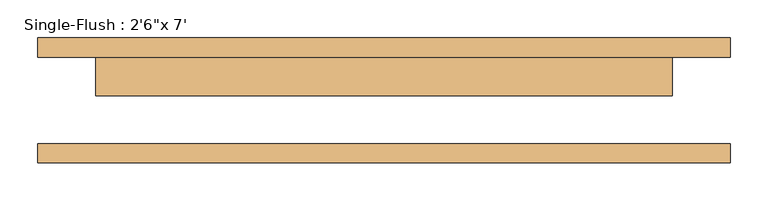
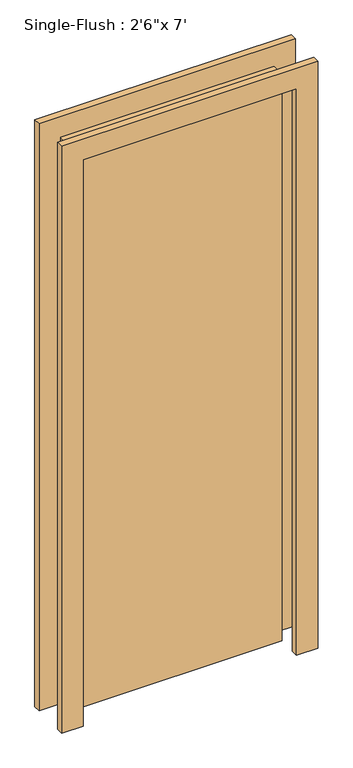
"""IFC4 building model written with IfcOpenShell, lengths in millimetres: door geometry."""

from ifc_helpers import new_model, si_unit, frame, origin, origin_with_axes, place, context, project, spatial, polyline, outline, extrude, source, transform, mapped, element, save


def door_214872d5(model_context):
    return source(origin(), model_context, "Body", "SweptSolid", [
        extrude(outline(polyline([(2209.8, -457.2), (0.0, -457.2), (0.0, -381.0), (2133.6, -381.0), (2133.6, 381.0), (0.0, 381.0), (0.0, 457.2), (2209.8, 457.2), (2209.8, -457.2)])), frame((0.0, 57.15, 0.0), z_axis=(0.0, 1.0, 0.0), x_axis=(0.0, 0.0, 1.0)), (0.0, 0.0, 1.0), 25.4),
        extrude(outline(polyline([(2209.8, 457.2), (2209.8, -457.2), (0.0, -457.2), (0.0, -381.0), (2133.6, -381.0), (2133.6, 381.0), (0.0, 381.0), (0.0, 457.2), (2209.8, 457.2)])), frame((0.0, -82.55, 0.0), z_axis=(0.0, 1.0, 0.0), x_axis=(0.0, 0.0, 1.0)), (0.0, 0.0, 1.0), 25.4),
        extrude(outline(polyline([(381.0, 6.35), (-381.0, 6.35), (-381.0, 57.15), (381.0, 57.15), (381.0, 6.35)])), origin_with_axes(), (0.0, 0.0, 1.0), 2133.6),
    ])


if __name__ == "__main__":
    model = new_model("IFC4")
    model_context = context("Model", 3, world=origin())
    ifc_project = project(units=[si_unit("LENGTHUNIT", "METRE", prefix="MILLI")], contexts=[model_context])
    site = spatial("IfcSite", under=ifc_project)
    building = spatial("IfcBuilding", under=site)
    placement = place(None, origin())
    door_shape = door_214872d5(model_context)
    element("IfcDoor", 1, ObjectType="Single-Flush : 2'6\"x 7'", at=placement, inside=building, context=model_context, shape_type="MappedRepresentation", body=[
        mapped(door_shape, transform((0.0, 0.0, 0.0), x_axis=(1.0, 0.0, 0.0), y_axis=(0.0, 1.0, 0.0), z_axis=(0.0, 0.0, 1.0))),
    ])
    save(model, "model.ifc")

# Revit data of these elements
# Type "Single-Flush : 2'6\"x 7'"
#   Type Mark = "8"
#   Construction Type Id = "MDOOR"
#   Assembly Code = "C1020"
#   Analytic Construction = "Metal"
#   Thickness = 0' - 2"
#   Heat Transfer Coefficient (U) = 0.651978 BTU/(h·ft²·°F)
#   Height = 7' - 0"
#   Trim Projection Ext = 0' - 1"
#   Trim Projection Int = 0' - 1"
#   Trim Width = 0' - 3"
#   Width = 2' - 6"
#   Define Thermal Properties by = 1
#   Door Material = Door - Panel
#   Frame Material = Door - Frame
#   Visual Light Transmittance = 0
#   Solar Heat Gain Coefficient = 0
#   Function = (empty or 0)
#   Wall Closure = (empty or 0)
# Element 1 (IfcDoor, "Single-Flush : 2'6\"x 7'")
#   Materials on its faces: "Door - Frame", "Door - Panel"
# Materials
#   "Door - Panel": class "Wood", colour RGB 210 159 95, transparency 0, Cost = 0
#   "Door - Frame": colour RGB 118 70 51, transparency 0, Cost = 0
